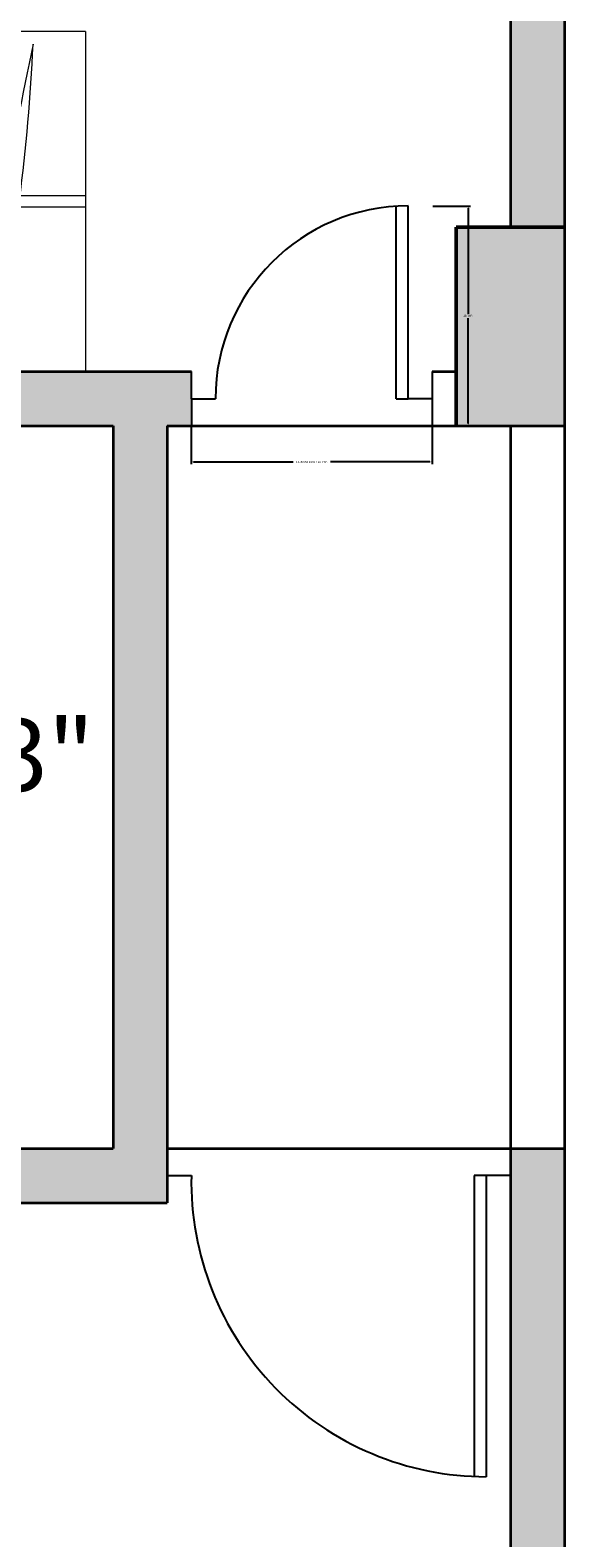
# Model space of a CAD drawing. Units: inches. Extents: x -28 to 485, y -861 to 54.
# Tile 9 of 14: x 116 to 162, y -240 to -115. Entities that reach past the tile are written whole.
import ezdxf

# ---------------------------------------------------------------- set-up
doc = ezdxf.new("R2010")
doc.units = ezdxf.units.IN
doc.header["$MEASUREMENT"] = 0
for name, color, linetype, lineweight in [('A-ANNO-DIMS', 2, 'Continuous', 18), ('A-AREA-IDEN', 7, 'Continuous', 18), ('A-COLS', 7, 'Continuous', 50), ('A-COLS-PATT', 8, 'Continuous', 13), ('A-DOOR', 3, 'Continuous', 25), ('A-FLOR-CASE', 8, 'Continuous', 18), ('A-WALL', 7, 'Continuous', 35), ('A-WALL-PATT', 34, 'Continuous', 13)]:
    doc.layers.add(name, color=color, linetype=linetype, lineweight=lineweight)
doc.styles.get("Standard").update_dxf_attribs({"font": 'arial.ttf'})
doc.dimstyles.get("Standard").update_dxf_attribs({"dimtxt": 0.18, "dimasz": 0.18, "dimexe": 0.18, "dimexo": 0.0625, "dimgap": 0.09, "dimtad": 0, "dimtih": 1, "dimtoh": 1, "dimdec": 0, "dimzin": 0, "dimdsep": 46, "dimlunit": 3, "dimtxsty": 'Standard', "dimcen": 0.09, "dimadec": 0, "dimazin": 0, "dimtfac": 1, "dimtdec": 0, "dimtofl": 0, "dimtmove": 0, "dimatfit": 3, "dimfxl": 1, "dimtolj": 1, "dimtzin": 0, "dimarcsym": 0})

# ---------------------------------------------------------------- blocks, each defined once
blk = doc.blocks.new('WARDROBE-HANGING')
for p, q in [((84.7, 28.23), (0, 28.23)), ((0, 28.23), (0, 0)), ((84.7, 28.23), (84.7, 0)), ((84.7, 14.59), (0, 14.59)), ((84.7, 13.65), (0, 13.65)), ((84.7, 0), (0, 0))]:
    blk.add_line(p, q)
for centre, start, end in [((153.74, 13.55), 175.0028, 184.9972), ((-142.25, 13.55), 355.0028, 4.9972), ((157.93, 13.55), 175.0028, 184.9972), ((-138.07, 13.55), 355.0028, 4.9972), ((-131.46, 33.65), 347.508, 357.5023), ((162.01, -4.96), 167.508, 177.5023), ((169.76, 14.46), 175.0028, 184.9972), ((-126.23, 14.46), 355.0028, 4.9972), ((174.85, 13.55), 175.0028, 184.9972), ((-121.15, 13.55), 355.0028, 4.9972), ((179.03, 13.55), 175.0028, 184.9972), ((-116.97, 13.55), 355.0028, 4.9972), ((-110.36, 33.65), 347.508, 357.5023), ((183.11, -4.96), 167.508, 177.5023), ((190.86, 14.46), 175.0028, 184.9972), ((-105.13, 14.46), 355.0028, 4.9972), ((196.03, 13.55), 175.0028, 184.9972), ((-99.97, 13.55), 355.0028, 4.9972), ((200.21, 13.55), 175.0028, 184.9972), ((-95.78, 13.55), 355.0028, 4.9972), ((204.29, -4.96), 167.508, 177.5023), ((-89.17, 33.65), 347.508, 357.5023), ((212.05, 14.46), 175.0028, 184.9972), ((-83.95, 14.46), 355.0028, 4.9972), ((217.13, 13.55), 175.0028, 184.9972), ((-78.86, 13.55), 355.0028, 4.9972), ((221.31, 13.55), 175.0028, 184.9972), ((-74.68, 13.55), 355.0028, 4.9972), ((225.4, -4.96), 167.508, 177.5023), ((-68.07, 33.65), 347.508, 357.5023)]:
    blk.add_arc(centre, 148.56, start, end)
blk = doc.blocks.new('DOOR-SWING-NARROW')
for p, q in [((17, 2.25), (17, 18.25)), ((18, 2.25), (18, 18.25)), ((0, 2.25), (0, 4.5)), ((20, 4.5), (20, 0)), ((0, 2.25), (0, 0)), ((0, 2.25), (2, 2.25)), ((17, 2.25), (18, 2.25)), ((20, 2.25), (18, 2.25))]:
    blk.add_line(p, q)
blk.add_arc((18, 2.25), 16, 90, 180)
blk = doc.blocks.new('*D36')
at = {"layer": 'A-ANNO-DIMS', "color": 0, "lineweight": -2, "transparency": 16777216}
for p, q in [((129.78, -147.43), (129.78, -150.55)), ((149.78, -147.43), (149.78, -150.55)), ((129.96, -150.37), (138.24, -150.37)), ((149.6, -150.37), (141.33, -150.37))]:
    blk.add_line(p, q, dxfattribs=at)
at = {"layer": 'A-ANNO-DIMS', "color": 0, "transparency": 16777216}
for points in [[(129.96, -150.34), (129.96, -150.4), (129.78, -150.37)], [(149.6, -150.34), (149.6, -150.4), (149.78, -150.37)]]:
    blk.add_solid(points, dxfattribs=at)
at = {"layer": 'Defpoints', "color": 0, "transparency": 16777216}
for p in [(129.78, -147.37), (149.78, -147.37), (149.78, -150.37)]:
    blk.add_point(p, dxfattribs=at)
at = {"layer": 'A-ANNO-DIMS', "color": 0, "transparency": 16777216, "insert": (139.78, -150.37), "char_height": 0.18, "attachment_point": 5}
blk.add_mtext('\\A1;NARROW DOOR 20 TYP.', dxfattribs=at)
blk = doc.blocks.new('*D37')
at = {"layer": 'A-ANNO-DIMS', "color": 0, "lineweight": -2, "transparency": 16777216}
for p, q in [((149.85, -129.12), (152.96, -129.12)), ((152.78, -129.3), (152.78, -138.06)), ((152.78, -147.19), (152.78, -138.42)), ((149.85, -147.37), (152.96, -147.37))]:
    blk.add_line(p, q, dxfattribs=at)
at = {"layer": 'A-ANNO-DIMS', "color": 0, "transparency": 16777216}
for points in [[(152.75, -129.3), (152.81, -129.3), (152.78, -129.12)], [(152.75, -147.19), (152.81, -147.19), (152.78, -147.37)]]:
    blk.add_solid(points, dxfattribs=at)
at = {"layer": 'Defpoints', "color": 0, "transparency": 16777216}
for p in [(149.78, -129.12), (152.78, -129.12), (149.78, -147.37)]:
    blk.add_point(p, dxfattribs=at)
at = {"layer": 'A-ANNO-DIMS', "color": 0, "transparency": 16777216, "insert": (152.78, -138.24), "char_height": 0.18, "attachment_point": 5}
blk.add_mtext('\\A1;18 TYP.', dxfattribs=at)

msp = doc.modelspace()

# ---------------------------------------------------------------- hatches: boundary and pattern name
at = {"layer": 'A-COLS-PATT'}
h = msp.add_hatch(color=256, dxfattribs=at)
h.dxf.hatch_style = 1
h.paths.add_polyline_path([(36.285, 10.133), (15.285, 10.133), (15.285, 1.133), (36.285, 1.133)])
h.paths.add_polyline_path([(160.785, 10.133), (139.785, 10.133), (139.785, 1.133), (160.785, 1.133)])
h.paths.add_polyline_path([(316.785, 10.133), (295.785, 10.133), (295.785, 1.133), (316.785, 1.133)])
h.paths.add_polyline_path([(441.285, 10.133), (420.285, 10.133), (420.285, 1.133), (441.285, 1.133)])
h.paths.add_polyline_path([(441.285, -138.367), (432.285, -138.367), (420.285, -138.367), (420.285, -147.367), (441.285, -147.367)])
h.paths.add_polyline_path([(304.785, -130.867), (295.785, -130.867), (295.785, -147.367), (304.785, -147.367), (304.785, -142.867)])
h.paths.add_polyline_path([(160.785, -130.867), (151.785, -130.867), (151.785, -142.867), (151.785, -147.367), (160.785, -147.367)])
h.paths.add_polyline_path([(36.285, -138.367), (24.285, -138.367), (15.285, -138.367), (15.285, -147.367), (36.285, -147.367)])
h.paths.add_polyline_path([(36.285, -355.867), (15.285, -355.867), (15.285, -364.867), (36.285, -364.867)])
h.paths.add_polyline_path([(160.785, -355.867), (139.785, -355.867), (139.785, -364.867), (160.785, -364.867)])
h.paths.add_polyline_path([(316.785, -355.867), (300.285, -355.867), (295.785, -355.867), (295.785, -364.867), (316.785, -364.867)])
at = {"layer": 'A-WALL-PATT'}
h = msp.add_hatch(color=256, dxfattribs=at)
h.dxf.hatch_style = 1
h.paths.add_polyline_path([(160.785, -808.867), (160.785, -817.867), (295.785, -817.867), (295.785, -808.867)])
h.paths.add_polyline_path([(316.785, -817.867), (323.776, -817.867), (323.776, -808.867), (316.785, -808.867)])
h.paths.add_polyline_path([(420.285, -817.867), (420.285, -808.867), (383.776, -808.867), (383.776, -817.867)])
h.paths.add_polyline_path([(432.285, -808.867), (441.285, -808.867), (441.285, -702.966), (432.285, -702.966), (432.285, -708.367), (397.785, -708.367), (397.785, -710.617), (397.785, -712.867), (432.285, -712.867)])
h.paths.add_polyline_path([(300.285, -712.867), (329.285, -712.867), (329.285, -710.617), (329.285, -708.367), (295.785, -708.367), (295.785, -808.867), (300.285, -808.867)])
h.paths.add_polyline_path([(160.785, -698.867), (158.535, -698.867), (156.285, -698.867), (156.285, -808.867), (160.785, -808.867)])
h.paths.add_polyline_path([(36.285, -808.867), (36.285, -817.867), (79.721, -817.867), (79.721, -808.867)])
h.paths.add_polyline_path([(15.285, -808.867), (24.285, -808.867), (24.285, -739.09), (15.285, -739.09)])
h.paths.add_polyline_path([(24.285, -640.781), (15.285, -640.781), (15.285, -679.09), (24.285, -679.09), (24.285, -664.867), (89.285, -664.867), (89.285, -662.617), (89.285, -660.367), (24.285, -660.367)])
h.paths.add_polyline_path([(15.285, -616.781), (24.285, -616.781), (24.285, -600.367), (15.285, -600.367)])
h.paths.add_polyline_path([(36.285, -595.867), (36.285, -600.367), (123.285, -600.367), (123.285, -660.367), (117.285, -660.367), (117.285, -664.867), (156.285, -664.867), (156.285, -670.867), (160.785, -670.867), (160.785, -660.367), (127.785, -660.367), (127.785, -600.367), (129.785, -600.367), (129.785, -598.117), (129.785, -595.867)])
h.paths.add_polyline_path([(367.785, -664.867), (363.285, -664.867), (363.285, -708.367), (357.285, -708.367), (357.285, -712.867), (369.785, -712.867), (369.785, -708.367), (367.785, -708.367)])
h.paths.add_polyline_path([(432.285, -664.867), (432.285, -666.966), (441.285, -666.966), (441.285, -642.367), (432.285, -642.367), (432.285, -660.367), (328.785, -660.367), (328.785, -664.867), (363.285, -664.867)])
h.paths.add_polyline_path([(333.285, -600.367), (420.285, -600.367), (420.285, -595.867), (326.785, -595.867), (326.785, -600.367), (328.785, -600.367), (328.785, -630.367), (331.035, -630.367), (333.285, -630.367)])
h.paths.add_polyline_path([(441.285, -600.367), (432.285, -600.367), (432.285, -618.367), (441.285, -618.367)])
h.paths.add_polyline_path([(432.285, -591.367), (441.285, -591.367), (441.285, -547.793), (432.285, -547.793)])
h.paths.add_polyline_path([(295.785, -588.367), (300.238, -588.367), (300.285, -583.867), (300.285, -451.867), (295.785, -451.867)])
h.paths.add_polyline_path([(420.285, -451.867), (420.285, -442.867), (316.785, -442.867), (316.785, -451.867)])
h.paths.add_polyline_path([(432.285, -487.793), (441.285, -487.793), (441.285, -451.867), (432.285, -451.867)])
h.paths.add_polyline_path([(432.285, -442.867), (441.285, -442.867), (441.285, -364.867), (432.285, -364.867)])
h.paths.add_polyline_path([(261.785, -451.867), (261.785, -447.367), (261.785, -444.758), (261.785, -442.867), (160.785, -442.867), (160.785, -451.867)])
h.paths.add_polyline_path([(139.785, -451.867), (139.785, -442.867), (36.285, -442.867), (36.285, -451.867)])
h.paths.add_polyline_path([(15.285, -491.617), (24.285, -491.617), (24.285, -451.867), (15.285, -451.867)])
h.paths.add_polyline_path([(24.285, -551.617), (15.285, -551.617), (15.285, -591.367), (24.285, -591.367)])
h.paths.add_polyline_path([(160.785, -451.867), (156.285, -451.867), (156.285, -588.367), (160.785, -588.367)])
h.paths.add_polyline_path([(139.785, -364.867), (139.785, -355.867), (36.285, -355.867), (36.285, -364.867)])
h.paths.add_polyline_path([(24.285, -364.867), (15.285, -364.867), (15.285, -373.867), (24.285, -373.867)])
h.paths.add_polyline_path([(15.285, -433.867), (15.285, -442.867), (24.285, -442.867), (24.285, -433.867)])
h.paths.add_polyline_path([(261.785, -364.867), (261.785, -360.367), (261.785, -355.867), (160.785, -355.867), (160.785, -364.867)])
h.paths.add_polyline_path([(295.785, -355.867), (289.785, -355.867), (289.785, -364.867), (295.785, -364.867)])
h.paths.add_polyline_path([(295.785, -355.867), (300.285, -355.867), (300.285, -259.867), (333.285, -259.867), (333.285, -257.617), (333.285, -255.367), (300.285, -255.367), (300.285, -207.367), (295.785, -207.367)])
h.paths.add_polyline_path([(420.285, -364.867), (420.285, -355.867), (316.785, -355.867), (316.785, -364.867)])
h.paths.add_polyline_path([(24.285, -311.192), (15.285, -311.192), (15.285, -355.867), (24.285, -355.867)])
h.paths.add_polyline_path([(24.285, -211.867), (54.144, -211.867), (54.144, -207.367), (24.285, -207.367), (24.285, -187.772), (15.285, -187.772), (15.285, -251.192), (24.285, -251.192)])
h.paths.add_polyline_path([(82.144, -207.367), (82.144, -209.617), (82.144, -211.867), (127.785, -211.867), (127.785, -147.367), (129.785, -147.367), (129.785, -145.117), (129.785, -142.867), (36.285, -142.867), (36.285, -147.367), (123.285, -147.367), (123.285, -207.367)])
h.paths.add_polyline_path([(160.785, -207.367), (156.285, -207.367), (156.285, -355.867), (160.785, -355.867)])
h.paths.add_polyline_path([(24.285, 1.133), (15.285, 1.133), (15.285, -54.408), (24.285, -54.408)])
h.paths.add_polyline_path([(36.285, 10.133), (36.285, 1.133), (70.235, 1.133), (70.235, 10.133)])
h.paths.add_polyline_path([(15.285, -138.367), (24.285, -138.367), (24.285, -114.408), (15.285, -114.408)])
h.paths.add_polyline_path([(24.285, -147.367), (15.285, -147.367), (15.285, -163.772), (24.285, -163.772)])
h.paths.add_polyline_path([(156.285, -130.867), (160.785, -130.867), (160.785, 1.133), (156.285, 1.133)])
h.paths.add_polyline_path([(130.235, 1.133), (139.785, 1.133), (139.785, 10.133), (130.235, 10.133)])
h.paths.add_polyline_path([(316.785, 10.133), (316.785, 1.133), (328.097, 1.133), (328.097, 10.133)])
h.paths.add_polyline_path([(300.285, 1.133), (295.785, 1.133), (295.785, -130.867), (300.285, -130.867)])
h.paths.add_polyline_path([(420.285, -147.367), (420.285, -142.867), (326.785, -142.867), (326.785, -145.117), (326.785, -147.367), (328.785, -147.367), (328.785, -177.367), (331.035, -177.367), (333.285, -177.367), (333.285, -147.367)])
h.paths.add_polyline_path([(333.285, -207.367), (333.285, -205.367), (328.785, -205.367), (328.785, -211.867), (363.285, -211.867), (363.285, -255.367), (361.285, -255.367), (361.285, -259.867), (369.785, -259.867), (369.785, -255.367), (367.785, -255.367), (367.785, -211.867), (432.285, -211.867), (432.285, -214.893), (441.285, -214.893), (441.285, -188.008), (432.285, -188.008), (432.285, -207.367)])
h.paths.add_polyline_path([(441.285, -250.893), (432.285, -250.893), (432.285, -255.367), (397.785, -255.367), (397.785, -257.617), (397.785, -259.867), (432.285, -259.867), (432.285, -355.867), (441.285, -355.867)])
h.paths.add_polyline_path([(432.285, -138.367), (441.285, -138.367), (441.285, -115.099), (432.285, -115.099)])
h.paths.add_polyline_path([(441.285, -147.367), (432.285, -147.367), (432.285, -164.008), (441.285, -164.008)])
h.paths.add_polyline_path([(420.285, 1.133), (420.285, 10.133), (388.097, 10.133), (388.097, 1.133)])
h.paths.add_polyline_path([(432.285, -55.099), (441.285, -55.099), (441.285, 1.133), (432.285, 1.133)])

# ---------------------------------------------------------------- linework, layer by layer
at = {"layer": 'A-COLS'}
for p, q in [((151.785, -142.867), (151.785, -130.867)), ((151.785, -130.867), (160.785, -130.867)), ((151.785, -147.367), (151.785, -142.867))]:
    msp.add_line(p, q, dxfattribs=at)
at = {"layer": 'A-DOOR'}
for p, q in [((127.785, -209.617), (129.785, -209.617)), ((153.285, -209.617), (153.285, -234.617)), ((154.285, -209.617), (153.285, -209.617)), ((156.285, -209.617), (154.285, -209.617)), ((154.285, -209.617), (154.285, -234.617))]:
    msp.add_line(p, q, dxfattribs=at)
msp.add_arc((154.285, -210.112), 24.505, 178.84255, 270, dxfattribs=at)
at = {"layer": 'A-WALL'}
for p, q in [((160.785, 10.133), (160.785, -364.867)), ((156.285, 1.133), (156.285, -130.867)), ((36.285, -142.867), (129.785, -142.867)), ((149.785, -142.867), (151.785, -142.867)), ((15.285, -147.367), (123.285, -147.367)), ((123.285, -147.367), (123.285, -207.367)), ((127.785, -147.367), (127.785, -211.867)), ((127.785, -147.367), (160.785, -147.367)), ((156.285, -147.367), (156.285, -355.867)), ((24.285, -207.367), (123.285, -207.367)), ((127.785, -207.367), (160.785, -207.367)), ((24.285, -211.867), (127.785, -211.867))]:
    msp.add_line(p, q, dxfattribs=at)

# ---------------------------------------------------------------- block references
at = {"layer": 'A-DOOR'}
msp.add_blockref('DOOR-SWING-NARROW', (129.785, -147.367), dxfattribs=at)
at = {"layer": 'A-FLOR-CASE'}
msp.add_blockref('WARDROBE-HANGING', (36.285, -142.867), dxfattribs=at)

# ---------------------------------------------------------------- texts
at = {"layer": 'A-AREA-IDEN', "insert": (86.556, -161.696), "char_height": 6, "attachment_point": 1}
msp.add_mtext_dynamic_manual_height_columns('TOILET\\P5\'0"X8\'3"', width=0.22148, gutter_width=1, heights=[0], dxfattribs=at)

# ---------------------------------------------------------------- dimensions: what is measured, and where the dimension line sits
at = {"layer": 'A-ANNO-DIMS'}
dim = msp.add_linear_dim(base=(152.785, -129.117), p1=(149.785, -147.367), p2=(149.785, -129.117), angle=90, text='<> TYP.', dimstyle='Standard', override={"dimdec": 0, "dimlfac": 1, "dimrnd": 0, "dimzin": 0, "dimdsep": 46, "dimlunit": 2}, dxfattribs=at)
dim.commit()
dim.dimension.update_dxf_attribs({"geometry": '*D37', "text_midpoint": (152.785, -138.242)})
dim = msp.add_linear_dim(base=(149.785, -150.367), p1=(129.785, -147.367), p2=(149.785, -147.367), text='NARROW DOOR <> TYP.', dimstyle='Standard', override={"dimdec": 0, "dimlfac": 1, "dimrnd": 0, "dimzin": 0, "dimdsep": 46, "dimlunit": 2}, dxfattribs=at)
dim.commit()
dim.dimension.update_dxf_attribs({"geometry": '*D36', "text_midpoint": (139.785, -150.367)})

doc.saveas('drawing.dxf')
